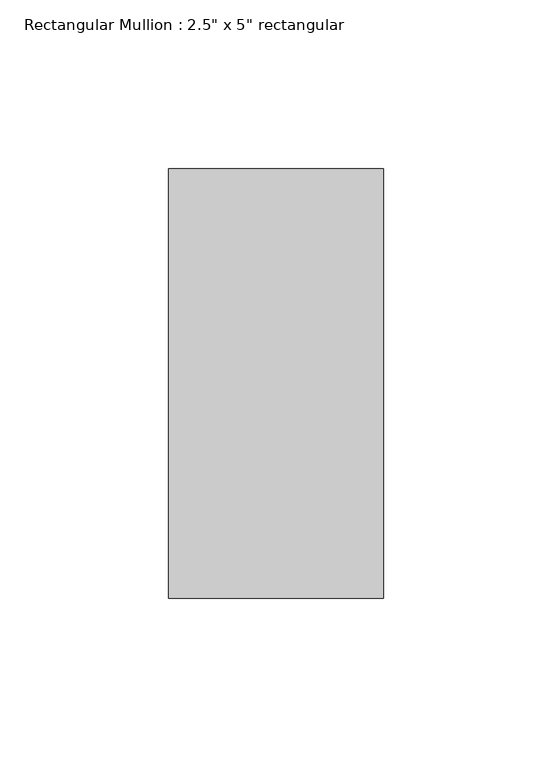
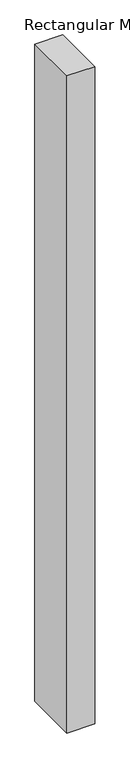
"""IFC4 building model written with IfcOpenShell, lengths in millimetres: member geometry."""

from ifc_helpers import new_model, si_unit, frame, origin, place, context, project, spatial, polyline, outline, extrude, source, transform, mapped, element, save


def member_cda0aa81(model_context):
    return source(origin(), model_context, "Body", "SweptSolid", [
        extrude(outline(polyline([(31.75, 63.5), (31.75, -63.5), (-31.75, -63.5), (-31.75, 63.5), (31.75, 63.5)])), frame((0.0, 0.0, -1587.5291864), z_axis=(0.0, 0.0, 1.0), x_axis=(1.0, 0.0, 0.0)), (0.0, 0.0, 1.0), 1587.5291864),
    ])


if __name__ == "__main__":
    model = new_model("IFC4")
    model_context = context("Model", 3, world=origin())
    ifc_project = project(units=[si_unit("LENGTHUNIT", "METRE", prefix="MILLI")], contexts=[model_context])
    site = spatial("IfcSite", under=ifc_project)
    building = spatial("IfcBuilding", under=site)
    placement = place(None, origin())
    member_shape = member_cda0aa81(model_context)
    element("IfcMember", 1, ObjectType="Rectangular Mullion : 2.5\" x 5\" rectangular", at=placement, inside=building, context=model_context, shape_type="MappedRepresentation", body=[
        mapped(member_shape, transform((0.0, 0.0, 0.0), x_axis=(1.0, 0.0, 0.0), y_axis=(0.0, 1.0, 0.0), z_axis=(0.0, 0.0, 1.0))),
    ])
    save(model, "model.ifc")

# Revit data of these elements
# Type "Rectangular Mullion : 2.5\" x 5\" rectangular"
#   built-in parameter 1007304 = 0.416667 (stored number, unit not read)
#   built-in parameter 1007301 = 0.104167 (stored number, unit not read)
#   built-in parameter 1007300 = 0.104167 (stored number, unit not read)
# Element 1 (IfcMember, "Rectangular Mullion : 2.5\" x 5\" rectangular")
#   Materials on its faces: "Aluminum"
# Materials
#   "Aluminum": class "Metal", colour RGB 247 247 247, transparency 0, Description = "Aluminum 6061", Cost = 0
